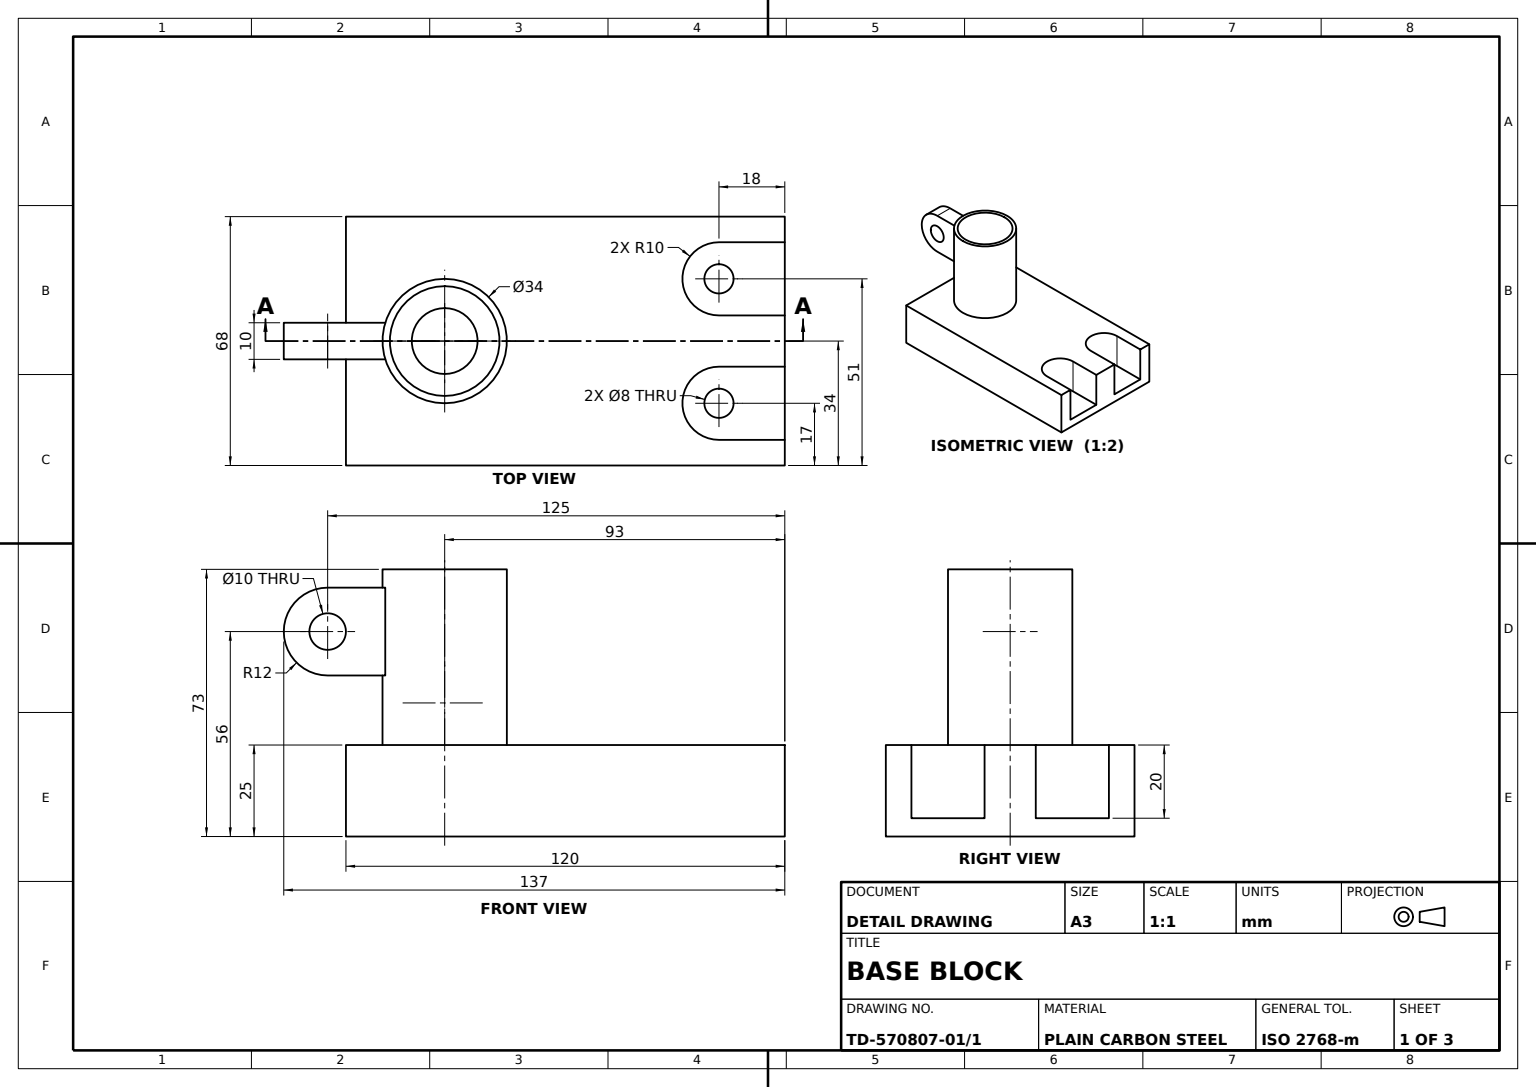
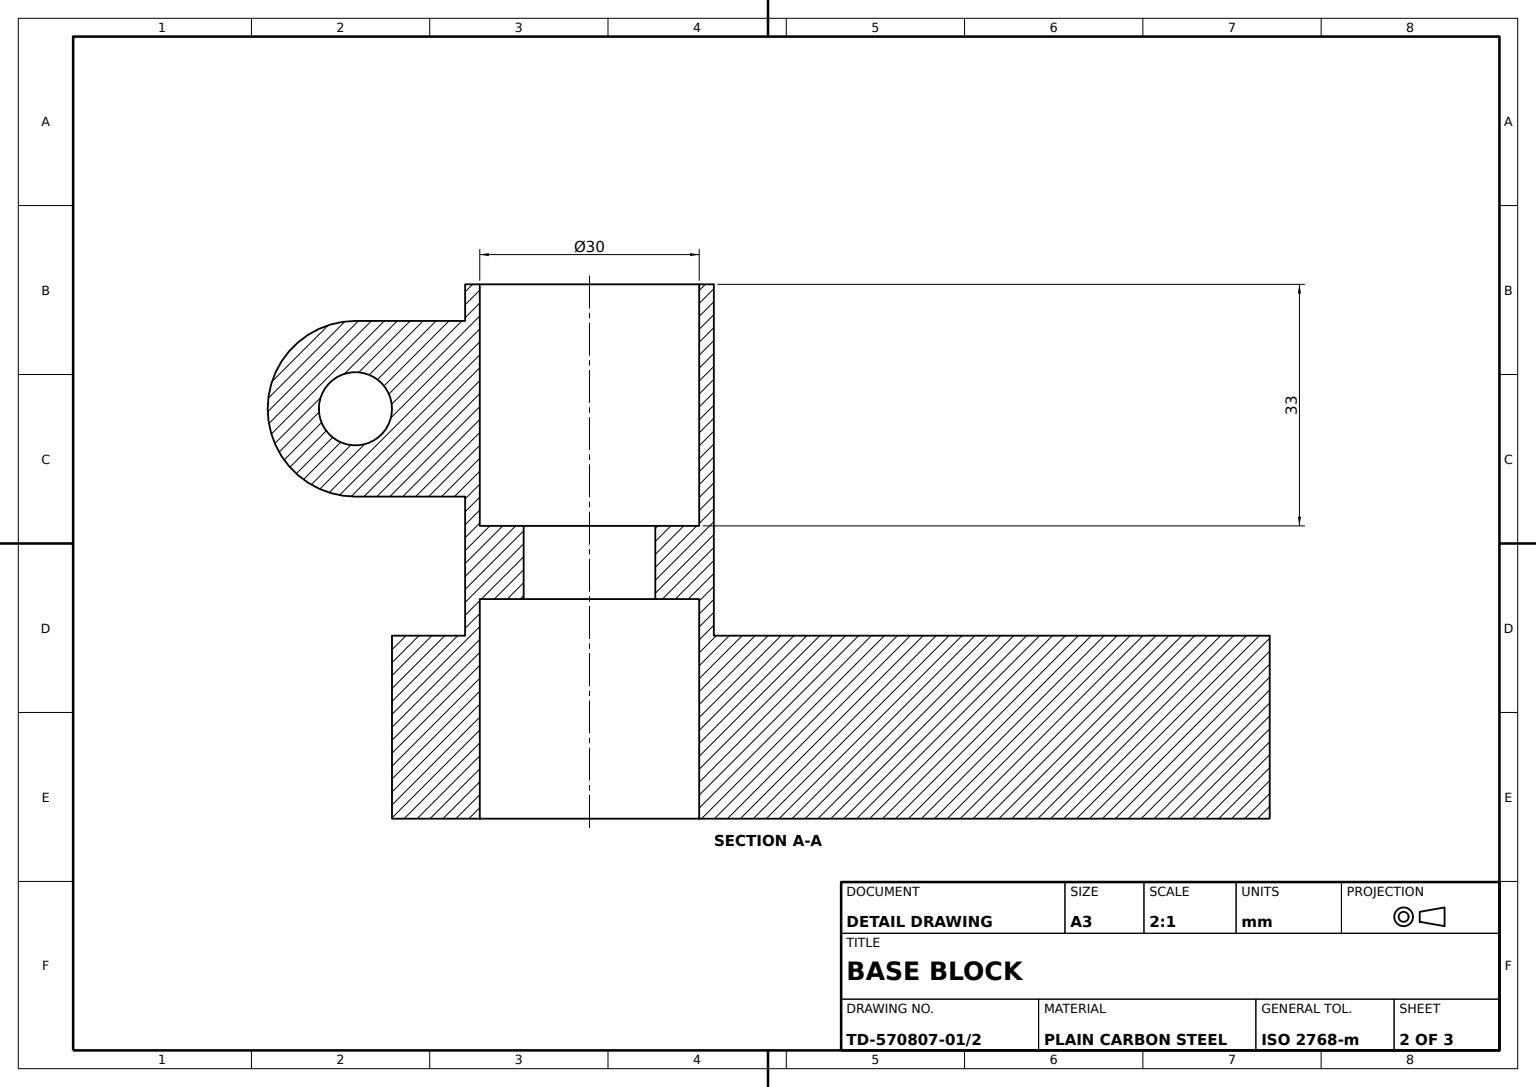
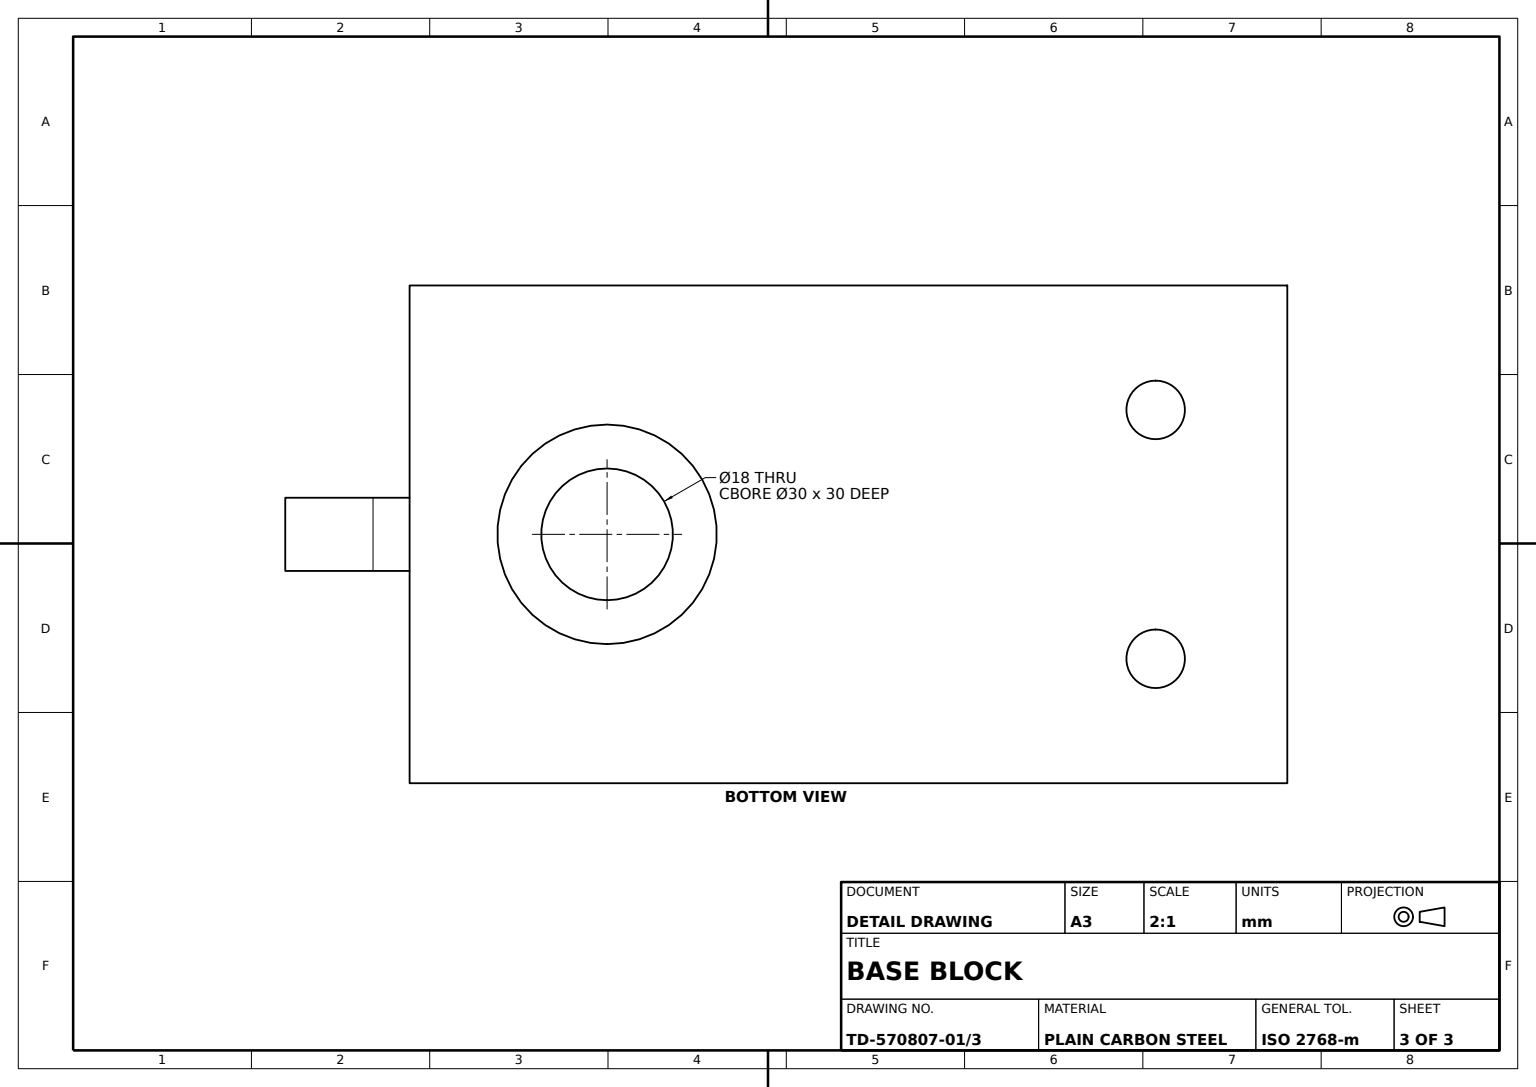
from build123d import *

# Parameters (mm, degrees)
BASE_PLATE_SKETCH_W       = 120
BASE_PLATE_SKETCH_H       = 68
BASE_PLATE_DEPTH          = 25
HUB_SKETCH_R              = 17
HUB_34_DEPTH              = 48
LUG_DEPTH                 = 5
HUB_BORE_SKETCH_R         = 15
HUB_BORE_30_DEPTH         = 33
THROUGH_HOLE_SKETCH_R     = 9
THROUGH_HOLE_18_DEPTH     = 10
BOTTOM_BORE_SKETCH_R      = 15
BOTTOM_BORE_30_DEPTH      = 95.519839187
LUG_HOLE_SKETCH_R         = 5
LUG_HOLE_10_DEPTH         = 25
MOUNTING_SLOTS_2X20_DEPTH = 20
SLOT_RELIEF_SKETCH_R      = 4
SLOT_RELIEF_CUTS_DEPTH    = 20


with BuildPart() as part:
    # Base Plate Sketch → Base Plate (new body)
    with BuildSketch(Plane(origin=(0, 0, 0), x_dir=(1, 0, 0), z_dir=(0, 1, 0))):
        Rectangle(BASE_PLATE_SKETCH_W, BASE_PLATE_SKETCH_H)
    extrude(amount=BASE_PLATE_DEPTH)

    # Hub Sketch → Hub Ø34 (add)
    with BuildSketch(Plane(origin=(0, 25, 0), x_dir=(1, 0, 0), z_dir=(0, 1, 0))):
        with Locations(Location((-33, 0, 0), (0, 0, 90))):
            Circle(HUB_SKETCH_R)
    extrude(amount=HUB_34_DEPTH)

    # Lug Sketch → Lug (add, symmetric)
    with BuildSketch(Plane.XY):
        with BuildLine():
            Line((-65, 68), (-48.898372545, 68))
            Line((-48.898372545, 68), (-48.898372545, 44))
            Line((-48.898372545, 44), (-65, 44))
            ThreePointArc((-65, 44), (-77, 56), (-65, 68))
        make_face()
    extrude(amount=LUG_DEPTH, both=True)

    # Hub Bore Sketch → Hub Bore Ø30 (cut)
    with BuildSketch(Plane(origin=(0, 73, 0), x_dir=(1, 0, 0), z_dir=(0, 1, 0))):
        with Locations(Location((-33, 0, 0), (0, 0, 270))):
            Circle(HUB_BORE_SKETCH_R)
    extrude(amount=-HUB_BORE_30_DEPTH, mode=Mode.SUBTRACT)

    # Through Hole Sketch → Through Hole Ø18 (cut)
    with BuildSketch(Plane(origin=(0, 40, 0), x_dir=(1, 0, 0), z_dir=(0, 1, 0))):
        with Locations(Location((-33, 0, 0), (0, 0, 270))):
            Circle(THROUGH_HOLE_SKETCH_R)
    extrude(amount=-THROUGH_HOLE_18_DEPTH, mode=Mode.SUBTRACT)

    # Bottom Bore Sketch → Bottom Bore Ø30 (cut, through all)
    with BuildSketch(Plane(origin=(0, 30, 0), x_dir=(1, 0, 0), z_dir=(0, 1, 0))):
        with Locations(Location((-33, 0, 0), (0, 0, 270))):
            Circle(BOTTOM_BORE_SKETCH_R)
    extrude(amount=-BOTTOM_BORE_30_DEPTH, mode=Mode.SUBTRACT)

    # Lug Hole Sketch → Lug Hole Ø10 (cut)
    with BuildSketch(Plane.XY.offset(5)):
        with Locations((-65, 56)):
            Circle(LUG_HOLE_SKETCH_R)
    extrude(amount=-LUG_HOLE_10_DEPTH, mode=Mode.SUBTRACT)

    # Mounting Slots Sketch → Mounting Slots 2x20 (cut)
    with BuildSketch(Plane(origin=(0, 25, 0), x_dir=(1, 0, 0), z_dir=(0, 1, 0))):
        with BuildLine():
            Line((42, 27), (60, 27))
            Line((60, 27), (60, 7))
            Line((60, 7), (42, 7))
            ThreePointArc((42, 7), (32, 17), (42, 27))
        make_face()
        with BuildLine():
            Line((42, -7), (60, -7))
            Line((60, -7), (60, -27))
            Line((60, -27), (42, -27))
            ThreePointArc((42, -27), (32, -17), (42, -7))
        make_face()
    extrude(amount=-MOUNTING_SLOTS_2X20_DEPTH, mode=Mode.SUBTRACT)

    # Slot Relief Sketch → Slot Relief Cuts (cut)
    with BuildSketch(Plane(origin=(0, 5, 0), x_dir=(1, 0, 0), z_dir=(0, 1, 0))):
        with Locations(Location((42, 17, 0), (0, 0, 270))):
            Circle(SLOT_RELIEF_SKETCH_R)
        with Locations(Location((42, -17, 0), (0, 0, 270))):
            Circle(SLOT_RELIEF_SKETCH_R)
    extrude(amount=-SLOT_RELIEF_CUTS_DEPTH, mode=Mode.SUBTRACT)


solid = part.part
